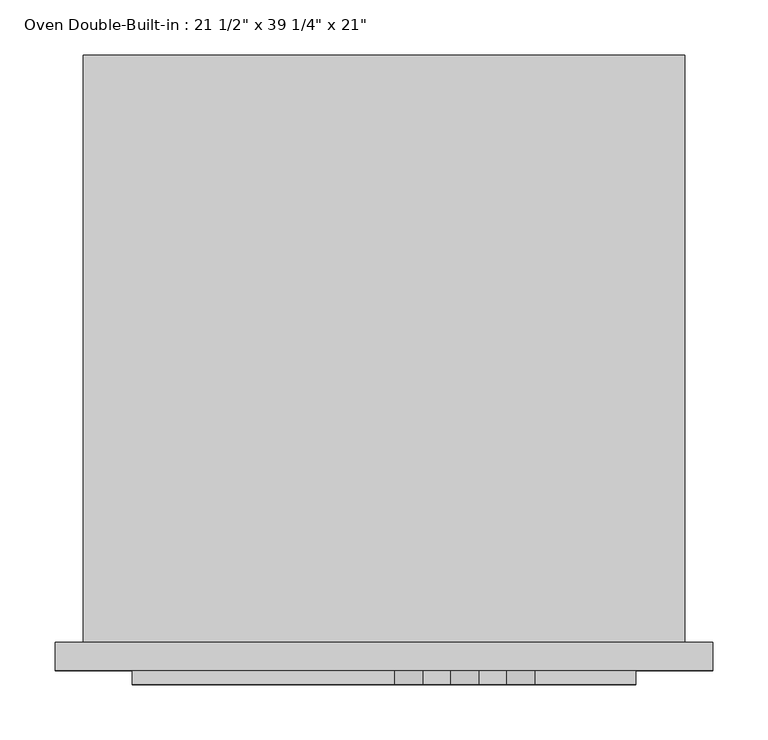
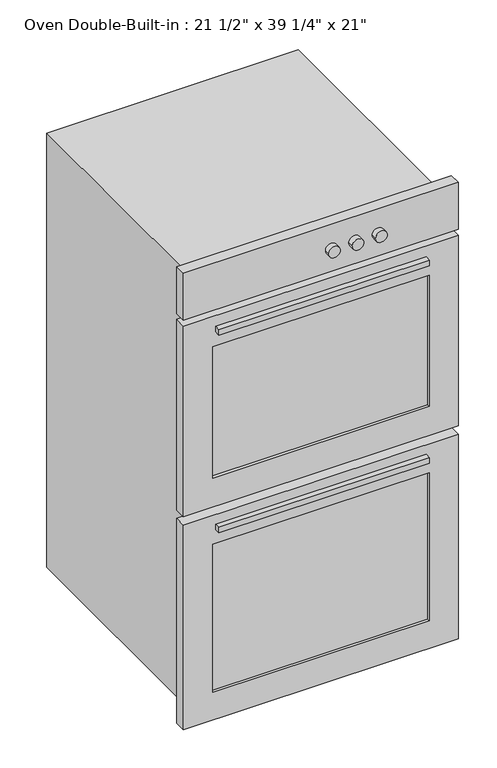
"""IFC4 building model written with IfcOpenShell, lengths in millimetres: proxy geometry."""

from ifc_helpers import new_model, si_unit, point, frame, frame_2d, origin, place, context, project, spatial, polyline, circle_curve, trimmed, segment, composite_curve, outline, extrude, source, transform, mapped, element, save


def proxy_8b8c2dc4(model_context):
    return source(origin(), model_context, "Body", "SweptSolid", [
        extrude(outline(polyline([(212.4750727, -100.2341411), (-282.8249273, -100.2341411), (-282.8249273, 382.3658589), (212.4750727, 382.3658589), (212.4750727, -100.2341411)])), frame((0.0, 0.0, 800.1), z_axis=(0.0, 0.0, 1.0), x_axis=(1.0, 0.0, 0.0)), (0.0, 0.0, 1.0), 19.05),
        extrude(outline(polyline([(212.4750727, -125.6341411), (-282.8249273, -125.6341411), (-282.8249273, -100.2341411), (212.4750727, -100.2341411), (212.4750727, -125.6341411)])), frame((0.0, 0.0, 1231.9720137), z_axis=(0.0, 0.0, 1.0), x_axis=(1.0, 0.0, 0.0)), (0.0, 0.0, 1.0), 95.1779863),
        extrude(outline(polyline([(212.4750727, -125.6341411), (-282.8249273, -125.6341411), (-282.8249273, -100.2341411), (212.4750727, -100.2341411), (212.4750727, -125.6341411)])), frame((0.0, 0.0, 768.35), z_axis=(0.0, 0.0, 1.0), x_axis=(1.0, 0.0, 0.0)), (0.0, 0.0, 1.0), 82.55),
        extrude(outline(composite_curve([segment(trimmed(circle_curve(frame_2d((1322.271693, -12.6998447)), 12.7), [point((1322.271693, -25.3998447))], [point((1322.271693, 0.0001553))], False, "CARTESIAN"), True, "CONTINUOUS"), segment(trimmed(circle_curve(frame_2d((1322.271693, -12.6998447)), 12.7), [point((1322.271693, 0.0001553))], [point((1322.271693, -25.3998447))], False, "CARTESIAN"), True, "CONTINUOUS")], self_intersect=False)), frame((0.0, -163.7341411, 0.0), z_axis=(0.0, 1.0, 0.0), x_axis=(0.0, 0.0, 1.0)), (0.0, 0.0, 1.0), 12.7),
        extrude(outline(composite_curve([segment(trimmed(circle_curve(frame_2d((1322.271693, 38.1001553)), 12.7), [point((1322.271693, 25.4001553))], [point((1322.271693, 50.8001553))], False, "CARTESIAN"), True, "CONTINUOUS"), segment(trimmed(circle_curve(frame_2d((1322.271693, 38.1001553)), 12.7), [point((1322.271693, 50.8001553))], [point((1322.271693, 25.4001553))], False, "CARTESIAN"), True, "CONTINUOUS")], self_intersect=False)), frame((0.0, -163.7341411, 0.0), z_axis=(0.0, 1.0, 0.0), x_axis=(0.0, 0.0, 1.0)), (0.0, 0.0, 1.0), 12.7),
        extrude(outline(composite_curve([segment(trimmed(circle_curve(frame_2d((1322.271693, 88.9001553)), 12.7), [point((1322.271693, 76.2001553))], [point((1322.271693, 101.6001553))], False, "CARTESIAN"), True, "CONTINUOUS"), segment(trimmed(circle_curve(frame_2d((1322.271693, 88.9001553)), 12.7), [point((1322.271693, 101.6001553))], [point((1322.271693, 76.2001553))], False, "CARTESIAN"), True, "CONTINUOUS")], self_intersect=False)), frame((0.0, -163.7341411, 0.0), z_axis=(0.0, 1.0, 0.0), x_axis=(0.0, 0.0, 1.0)), (0.0, 0.0, 1.0), 12.7),
        extrude(outline(polyline([(193.4250727, -163.7341411), (-263.7749273, -163.7341411), (-263.7749273, -151.0341411), (193.4250727, -151.0341411), (193.4250727, -163.7341411)])), frame((0.0, 0.0, 1219.2720137), z_axis=(0.0, 0.0, 1.0), x_axis=(1.0, 0.0, 0.0)), (0.0, 0.0, 1.0), 12.7),
        extrude(outline(polyline([(193.4250727, -163.7341411), (-263.7749273, -163.7341411), (-263.7749273, -151.0341411), (193.4250727, -151.0341411), (193.4250727, -163.7341411)])), frame((0.0, 0.0, 765.2470137), z_axis=(0.0, 0.0, 1.0), x_axis=(1.0, 0.0, 0.0)), (0.0, 0.0, 1.0), 12.7),
        extrude(outline(polyline([(199.7750727, -144.6841411), (-270.1249273, -144.6841411), (-270.1249273, -138.3341411), (199.7750727, -138.3341411), (199.7750727, -144.6841411)])), frame((0.0, 0.0, 885.825), z_axis=(0.0, 0.0, 1.0), x_axis=(1.0, 0.0, 0.0)), (0.0, 0.0, 1.0), 301.625),
        extrude(outline(polyline([(199.7750727, -144.6841411), (-270.1249273, -144.6841411), (-270.1249273, -138.3341411), (199.7750727, -138.3341411), (199.7750727, -144.6841411)])), frame((0.0, 0.0, 393.7), z_axis=(0.0, 0.0, 1.0), x_axis=(1.0, 0.0, 0.0)), (0.0, 0.0, 1.0), 339.725),
        extrude(outline(polyline([(263.2750727, -151.0341411), (-333.6249273, -151.0341411), (-333.6249273, -125.6341411), (263.2750727, -125.6341411), (263.2750727, -151.0341411)])), frame((0.0, 0.0, 1270.0), z_axis=(0.0, 0.0, 1.0), x_axis=(1.0, 0.0, 0.0)), (0.0, 0.0, 1.0), 107.95),
        extrude(outline(polyline([(1257.3, 263.2750727), (1257.3, -333.6249273), (819.15, -333.6249273), (819.15, 263.2750727), (1257.3, 263.2750727)]), holes=[polyline([(1187.45, 199.7750727), (885.825, 199.7750727), (885.825, -270.1249273), (1187.45, -270.1249273), (1187.45, 199.7750727)])]), frame((0.0, -151.0341411, 0.0), z_axis=(0.0, 1.0, 0.0), x_axis=(0.0, 0.0, 1.0)), (0.0, 0.0, 1.0), 25.4),
        extrude(outline(polyline([(800.1, 263.2750727), (800.1, -333.6249273), (330.2, -333.6249273), (330.2, 263.2750727), (800.1, 263.2750727)]), holes=[polyline([(733.425, 199.7750727), (393.7, 199.7750727), (393.7, -270.1249273), (733.425, -270.1249273), (733.425, 199.7750727)])]), frame((0.0, -151.0341411, 0.0), z_axis=(0.0, 1.0, 0.0), x_axis=(0.0, 0.0, 1.0)), (0.0, 0.0, 1.0), 25.4),
        extrude(outline(polyline([(212.4750727, 382.3658589), (-282.8249273, 382.3658589), (-282.8249273, 407.7658589), (212.4750727, 407.7658589), (212.4750727, 382.3658589)])), frame((0.0, 0.0, 381.0), z_axis=(0.0, 0.0, 1.0), x_axis=(1.0, 0.0, 0.0)), (0.0, 0.0, 1.0), 946.15),
        extrude(outline(polyline([(1352.55, 237.8750727), (1352.55, -308.2249273), (355.6, -308.2249273), (355.6, 237.8750727), (1352.55, 237.8750727)]), holes=[polyline([(1327.15, 212.4750727), (381.0, 212.4750727), (381.0, -282.8249273), (1327.15, -282.8249273), (1327.15, 212.4750727)])]), frame((0.0, -125.6341411, 0.0), z_axis=(0.0, 1.0, 0.0), x_axis=(0.0, 0.0, 1.0)), (0.0, 0.0, 1.0), 533.4),
    ])


if __name__ == "__main__":
    model = new_model("IFC4")
    model_context = context("Model", 3, world=origin())
    ifc_project = project(units=[si_unit("LENGTHUNIT", "METRE", prefix="MILLI")], contexts=[model_context])
    site = spatial("IfcSite", under=ifc_project)
    building = spatial("IfcBuilding", under=site)
    placement = place(None, origin())
    proxy_shape = proxy_8b8c2dc4(model_context)
    element("IfcBuildingElementProxy", 1, Name="Oven Double-Built-in : 21 1/2\" x 39 1/4\" x 21\"", ObjectType="Oven Double-Built-in : 21 1/2\" x 39 1/4\" x 21\"", at=placement, inside=building, context=model_context, shape_type="MappedRepresentation", body=[
        mapped(proxy_shape, transform((0.0, 0.0, 0.0), x_axis=(1.0, 0.0, 0.0), y_axis=(0.0, 1.0, 0.0), z_axis=(0.0, 0.0, 1.0))),
    ])
    save(model, "model.ifc")

# Revit data of these elements
# Type "Oven Double-Built-in : 21 1/2\" x 39 1/4\" x 21\""
#   Label = "OVEN"
#   Assembly Code = "E1090400"
#   Depth = 1' - 9"
#   Height = 3' - 3 1/4"
#   Width = 1' - 9 1/2"
#   Oven Material = Metal - Stainless Steel, Polished
#   Default Elevation = 0
# Element 1 (IfcBuildingElementProxy, "Oven Double-Built-in : 21 1/2\" x 39 1/4\" x 21\"")
#   Materials on its faces: "Steel", "Metal - Stainless Steel, Polished", "Glass"
# Materials
#   "Metal - Stainless Steel, Polished": class "Metal", colour RGB 216 216 216, transparency 0
#   "Steel": class "Metal", colour RGB 247 247 247, transparency 0, Description = "Steel, mill finish", Cost = 0
#   "Glass": class "Glass", colour RGB 0 128 192, transparency 0.75, Description = "Soda Lime Glass", Cost = 0
